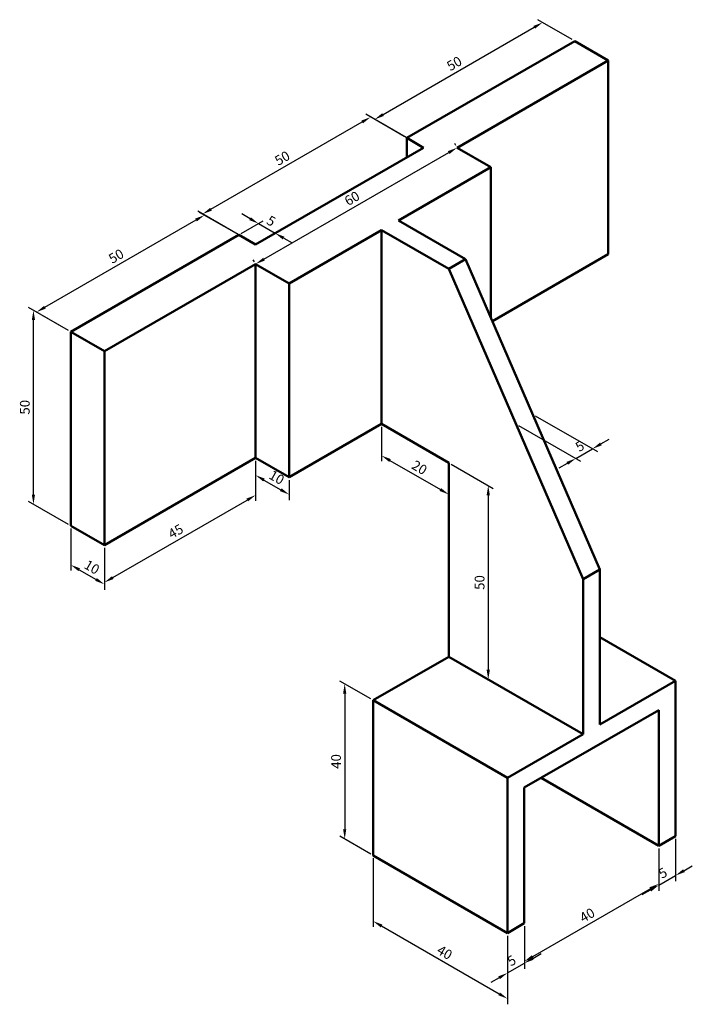
# Model space of a CAD drawing. Units: millimetres. Extents: x 2718 to 2891, y 1466 to 1720.
import ezdxf

# ---------------------------------------------------------------- set-up
doc = ezdxf.new("R2010")
doc.units = ezdxf.units.MM
doc.layers.add('M-DIMS', color=2, linetype='Continuous', lineweight=25)
doc.layers.add('M-OUTL', color=7, linetype='Continuous', lineweight=50)
doc.styles.get("Standard").update_dxf_attribs({"font": 'arial.ttf'})
doc.dimstyles.new('ISO-25', dxfattribs={"dimtxt": 2.5, "dimasz": 2.5, "dimexe": 1.25, "dimexo": 0.625, "dimtad": 1, "dimtxsty": 'Standard', "dimcen": 2.5, "dimadec": 0, "dimazin": 0, "dimtfac": 1, "dimtmove": 0, "dimatfit": 3, "dimfxl": 1, "dimarcsym": 0})

# ---------------------------------------------------------------- blocks, each defined once
blk = doc.blocks.new('*D1')
at = {"layer": 'Defpoints', "color": 0, "transparency": 16777216}
for p in [(2808.89, 1504.71), (2843.54, 1484.71), (2843.54, 1467.77)]:
    blk.add_point(p, dxfattribs=at)
at = {"layer": 'M-DIMS', "color": 0, "lineweight": -2, "transparency": 16777216}
for p, q in [((2808.89, 1503.99), (2808.89, 1486.33)), ((2811.06, 1486.52), (2841.37, 1469.02)), ((2843.54, 1483.99), (2843.54, 1466.33))]:
    blk.add_line(p, q, dxfattribs=at)
at = {"layer": 'M-DIMS', "color": 0, "transparency": 16777216}
for points in [[(2811.27, 1486.88), (2810.85, 1486.16), (2808.89, 1487.77)], [(2841.58, 1469.38), (2841.16, 1468.66), (2843.54, 1467.77)]]:
    blk.add_solid(points, dxfattribs=at)
at = {"layer": 'M-DIMS', "color": 0, "transparency": 16777216, "insert": (2827.17, 1479.42), "char_height": 2.5, "attachment_point": 5, "rotation": 330}
blk.add_mtext('40', dxfattribs=at)
blk = doc.blocks.new('*D2')
at = {"layer": 'Defpoints', "color": 0, "transparency": 16777216}
for p in [(2847.87, 1487.21), (2843.54, 1484.71), (2847.87, 1476.93)]:
    blk.add_point(p, dxfattribs=at)
at = {"layer": 'M-DIMS', "color": 0, "lineweight": -2, "transparency": 16777216}
for p, q in [((2847.87, 1486.49), (2847.87, 1475.49)), ((2843.54, 1483.99), (2843.54, 1472.99)), ((2850.03, 1478.18), (2852.2, 1479.43)), ((2843.54, 1474.43), (2847.87, 1476.93)), ((2841.37, 1473.18), (2839.21, 1471.93))]:
    blk.add_line(p, q, dxfattribs=at)
at = {"layer": 'M-DIMS', "color": 0, "transparency": 16777216}
for points in [[(2849.82, 1478.54), (2850.24, 1477.82), (2847.87, 1476.93)], [(2841.16, 1473.54), (2841.58, 1472.82), (2843.54, 1474.43)]]:
    blk.add_solid(points, dxfattribs=at)
at = {"layer": 'M-DIMS', "color": 0, "transparency": 16777216, "insert": (2844.75, 1477.32), "char_height": 2.5, "attachment_point": 5, "rotation": 30}
blk.add_mtext('5', dxfattribs=at)
blk = doc.blocks.new('*D3')
at = {"layer": 'Defpoints', "color": 0, "transparency": 16777216}
for p in [(2882.51, 1507.21), (2882.51, 1497.39), (2847.87, 1487.21)]:
    blk.add_point(p, dxfattribs=at)
at = {"layer": 'M-DIMS', "color": 0, "lineweight": -2, "transparency": 16777216}
for p, q in [((2882.51, 1506.49), (2882.51, 1495.95)), ((2850.03, 1478.64), (2880.34, 1496.14)), ((2847.87, 1486.49), (2847.87, 1475.95))]:
    blk.add_line(p, q, dxfattribs=at)
at = {"layer": 'M-DIMS', "color": 0, "transparency": 16777216}
for points in [[(2880.13, 1496.5), (2880.55, 1495.78), (2882.51, 1497.39)], [(2849.82, 1479), (2850.24, 1478.28), (2847.87, 1477.39)]]:
    blk.add_solid(points, dxfattribs=at)
at = {"layer": 'M-DIMS', "color": 0, "transparency": 16777216, "insert": (2864.24, 1489.04), "char_height": 2.5, "attachment_point": 5, "rotation": 30}
blk.add_mtext('40', dxfattribs=at)
blk = doc.blocks.new('*D4')
at = {"layer": 'Defpoints', "color": 0, "transparency": 16777216}
for p in [(2886.84, 1509.71), (2882.51, 1507.21), (2886.84, 1499.53)]:
    blk.add_point(p, dxfattribs=at)
at = {"layer": 'M-DIMS', "color": 0, "lineweight": -2, "transparency": 16777216}
for p, q in [((2886.84, 1508.99), (2886.84, 1498.08)), ((2882.51, 1506.49), (2882.51, 1495.58)), ((2889, 1500.78), (2891.17, 1502.03)), ((2882.51, 1497.03), (2886.84, 1499.53)), ((2880.34, 1495.78), (2878.18, 1494.53))]:
    blk.add_line(p, q, dxfattribs=at)
at = {"layer": 'M-DIMS', "color": 0, "transparency": 16777216}
for points in [[(2888.79, 1501.14), (2889.21, 1500.42), (2886.84, 1499.53)], [(2880.13, 1496.14), (2880.55, 1495.42), (2882.51, 1497.03)]]:
    blk.add_solid(points, dxfattribs=at)
at = {"layer": 'M-DIMS', "color": 0, "transparency": 16777216, "insert": (2883.72, 1499.92), "char_height": 2.5, "attachment_point": 5, "rotation": 30}
blk.add_mtext('5', dxfattribs=at)
blk = doc.blocks.new('*D5')
at = {"layer": 'Defpoints', "color": 0, "transparency": 16777216}
for p in [(2828.38, 1605.96), (2828.38, 1555.96), (2838.56, 1550.09)]:
    blk.add_point(p, dxfattribs=at)
at = {"layer": 'M-DIMS', "color": 0, "lineweight": -2, "transparency": 16777216}
for p, q in [((2829.01, 1605.6), (2839.81, 1599.36)), ((2838.56, 1597.59), (2838.56, 1552.59)), ((2829.01, 1555.6), (2839.81, 1549.36))]:
    blk.add_line(p, q, dxfattribs=at)
at = {"layer": 'M-DIMS', "color": 0, "transparency": 16777216}
for points in [[(2838.15, 1597.59), (2838.98, 1597.59), (2838.56, 1600.09)], [(2838.15, 1552.59), (2838.98, 1552.59), (2838.56, 1550.09)]]:
    blk.add_solid(points, dxfattribs=at)
at = {"layer": 'M-DIMS', "color": 0, "transparency": 16777216, "insert": (2836.66, 1575.09), "char_height": 2.5, "attachment_point": 5, "rotation": 90}
blk.add_mtext('50', dxfattribs=at)
blk = doc.blocks.new('*D6')
at = {"layer": 'Defpoints', "color": 0, "transparency": 16777216}
for p in [(2811.06, 1615.96), (2828.38, 1605.96), (2828.38, 1597.81)]:
    blk.add_point(p, dxfattribs=at)
at = {"layer": 'M-DIMS', "color": 0, "lineweight": -2, "transparency": 16777216}
for p, q in [((2811.06, 1615.24), (2811.06, 1606.37)), ((2813.22, 1606.56), (2826.22, 1599.06)), ((2828.38, 1605.24), (2828.38, 1596.37))]:
    blk.add_line(p, q, dxfattribs=at)
at = {"layer": 'M-DIMS', "color": 0, "transparency": 16777216}
for points in [[(2813.43, 1606.92), (2813.02, 1606.2), (2811.06, 1607.81)], [(2826.42, 1599.42), (2826.01, 1598.7), (2828.38, 1597.81)]]:
    blk.add_solid(points, dxfattribs=at)
at = {"layer": 'M-DIMS', "color": 0, "transparency": 16777216, "insert": (2820.67, 1604.46), "char_height": 2.5, "attachment_point": 5, "rotation": 330}
blk.add_mtext('20', dxfattribs=at)
blk = doc.blocks.new('*D7')
at = {"layer": 'Defpoints', "color": 0, "transparency": 16777216}
for p in [(2830.55, 1687.21), (2830.55, 1687.21), (2778.58, 1657.21)]:
    blk.add_point(p, dxfattribs=at)
at = {"layer": 'M-DIMS', "color": 0, "lineweight": -2, "transparency": 16777216}
for p, q in [((2780.75, 1658.46), (2828.38, 1685.96)), ((2830.23, 1687.76), (2829.92, 1688.3)), ((2778.27, 1657.76), (2777.96, 1658.3))]:
    blk.add_line(p, q, dxfattribs=at)
at = {"layer": 'M-DIMS', "color": 0, "transparency": 16777216}
for points in [[(2828.17, 1686.32), (2828.59, 1685.6), (2830.55, 1687.21)], [(2780.54, 1658.82), (2780.96, 1658.1), (2778.58, 1657.21)]]:
    blk.add_solid(points, dxfattribs=at)
at = {"layer": 'M-DIMS', "color": 0, "transparency": 16777216, "insert": (2803.61, 1673.86), "char_height": 2.5, "attachment_point": 5, "rotation": 30}
blk.add_mtext('60', dxfattribs=at)
blk = doc.blocks.new('*D8')
at = {"layer": 'Defpoints', "color": 0, "transparency": 16777216}
for p in [(2778.58, 1607.21), (2787.24, 1602.21), (2787.24, 1597.77)]:
    blk.add_point(p, dxfattribs=at)
at = {"layer": 'M-DIMS', "color": 0, "lineweight": -2, "transparency": 16777216}
for p, q in [((2778.58, 1606.49), (2778.58, 1601.33)), ((2780.75, 1601.52), (2785.08, 1599.02)), ((2787.24, 1601.49), (2787.24, 1596.33))]:
    blk.add_line(p, q, dxfattribs=at)
at = {"layer": 'M-DIMS', "color": 0, "transparency": 16777216}
for points in [[(2780.96, 1601.88), (2780.54, 1601.16), (2778.58, 1602.77)], [(2785.29, 1599.38), (2784.87, 1598.66), (2787.24, 1597.77)]]:
    blk.add_solid(points, dxfattribs=at)
at = {"layer": 'M-DIMS', "color": 0, "transparency": 16777216, "insert": (2783.86, 1601.92), "char_height": 2.5, "attachment_point": 5, "rotation": 330}
blk.add_mtext('10', dxfattribs=at)
blk = doc.blocks.new('*D9')
at = {"layer": 'Defpoints', "color": 0, "transparency": 16777216}
for p in [(2778.58, 1607.21), (2778.58, 1597.61), (2739.61, 1584.71)]:
    blk.add_point(p, dxfattribs=at)
at = {"layer": 'M-DIMS', "color": 0, "lineweight": -2, "transparency": 16777216}
for p, q in [((2778.58, 1606.49), (2778.58, 1596.16)), ((2741.78, 1576.36), (2776.42, 1596.36)), ((2739.61, 1583.99), (2739.61, 1573.66))]:
    blk.add_line(p, q, dxfattribs=at)
at = {"layer": 'M-DIMS', "color": 0, "transparency": 16777216}
for points in [[(2776.21, 1596.72), (2776.63, 1596), (2778.58, 1597.61)], [(2741.57, 1576.72), (2741.99, 1576), (2739.61, 1575.11)]]:
    blk.add_solid(points, dxfattribs=at)
at = {"layer": 'M-DIMS', "color": 0, "transparency": 16777216, "insert": (2758.15, 1588), "char_height": 2.5, "attachment_point": 5, "rotation": 30}
blk.add_mtext('45', dxfattribs=at)
blk = doc.blocks.new('*D10')
at = {"layer": 'Defpoints', "color": 0, "transparency": 16777216}
for p in [(2730.95, 1589.71), (2739.61, 1584.71), (2739.61, 1574.64)]:
    blk.add_point(p, dxfattribs=at)
at = {"layer": 'M-DIMS', "color": 0, "lineweight": -2, "transparency": 16777216}
for p, q in [((2730.95, 1588.99), (2730.95, 1578.19)), ((2739.61, 1583.99), (2739.61, 1573.19)), ((2733.12, 1578.39), (2737.45, 1575.89))]:
    blk.add_line(p, q, dxfattribs=at)
at = {"layer": 'M-DIMS', "color": 0, "transparency": 16777216}
for points in [[(2733.33, 1578.75), (2732.91, 1578.03), (2730.95, 1579.64)], [(2737.66, 1576.25), (2737.24, 1575.53), (2739.61, 1574.64)]]:
    blk.add_solid(points, dxfattribs=at)
at = {"layer": 'M-DIMS', "color": 0, "transparency": 16777216, "insert": (2736.23, 1578.78), "char_height": 2.5, "attachment_point": 5, "rotation": 330}
blk.add_mtext('10', dxfattribs=at)
blk = doc.blocks.new('*D11')
at = {"layer": 'Defpoints', "color": 0, "transparency": 16777216}
for p in [(2721.32, 1645.28), (2730.95, 1639.71), (2730.95, 1589.71)]:
    blk.add_point(p, dxfattribs=at)
at = {"layer": 'M-DIMS', "color": 0, "lineweight": -2, "transparency": 16777216}
for p, q in [((2730.33, 1640.07), (2720.07, 1646)), ((2721.32, 1597.78), (2721.32, 1642.78)), ((2730.33, 1590.07), (2720.07, 1596))]:
    blk.add_line(p, q, dxfattribs=at)
at = {"layer": 'M-DIMS', "color": 0, "transparency": 16777216}
for points in [[(2720.9, 1642.78), (2721.73, 1642.78), (2721.32, 1645.28)], [(2720.9, 1597.78), (2721.73, 1597.78), (2721.32, 1595.28)]]:
    blk.add_solid(points, dxfattribs=at)
at = {"layer": 'M-DIMS', "color": 0, "transparency": 16777216, "insert": (2719.42, 1620.28), "char_height": 2.5, "attachment_point": 5, "rotation": 90}
blk.add_mtext('50', dxfattribs=at)
blk = doc.blocks.new('*D12')
at = {"layer": 'Defpoints', "color": 0, "transparency": 16777216}
for p in [(2765.41, 1669.82), (2774.25, 1664.71), (2730.95, 1639.71)]:
    blk.add_point(p, dxfattribs=at)
at = {"layer": 'M-DIMS', "color": 0, "lineweight": -2, "transparency": 16777216}
for p, q in [((2724.27, 1646.07), (2763.24, 1668.57)), ((2773.63, 1665.07), (2764.16, 1670.54)), ((2730.33, 1640.07), (2720.86, 1645.54))]:
    blk.add_line(p, q, dxfattribs=at)
at = {"layer": 'M-DIMS', "color": 0, "transparency": 16777216}
for points in [[(2763.03, 1668.93), (2763.45, 1668.21), (2765.41, 1669.82)], [(2724.06, 1646.43), (2724.48, 1645.71), (2722.11, 1644.82)]]:
    blk.add_solid(points, dxfattribs=at)
at = {"layer": 'M-DIMS', "color": 0, "transparency": 16777216, "insert": (2742.81, 1658.97), "char_height": 2.5, "attachment_point": 5, "rotation": 30}
blk.add_mtext('50', dxfattribs=at)
blk = doc.blocks.new('*D13')
at = {"layer": 'Defpoints', "color": 0, "transparency": 16777216}
for p in [(2774.25, 1664.71), (2783.66, 1665.14), (2778.58, 1662.21)]:
    blk.add_point(p, dxfattribs=at)
at = {"layer": 'M-DIMS', "color": 0, "lineweight": -2, "transparency": 16777216}
for p, q in [((2774.88, 1665.07), (2780.58, 1668.37)), ((2777.17, 1668.89), (2775, 1670.14)), ((2779.21, 1662.57), (2784.91, 1665.87)), ((2779.33, 1667.64), (2783.66, 1665.14)), ((2785.83, 1663.89), (2787.99, 1662.64))]:
    blk.add_line(p, q, dxfattribs=at)
at = {"layer": 'M-DIMS', "color": 0, "transparency": 16777216}
for points in [[(2777.37, 1669.26), (2776.96, 1668.53), (2779.33, 1667.64)], [(2786.03, 1664.26), (2785.62, 1663.53), (2783.66, 1665.14)]]:
    blk.add_solid(points, dxfattribs=at)
at = {"layer": 'M-DIMS', "color": 0, "transparency": 16777216, "insert": (2782.44, 1668.04), "char_height": 2.5, "attachment_point": 5, "rotation": 330}
blk.add_mtext('5', dxfattribs=at)
blk = doc.blocks.new('*D14')
at = {"layer": 'Defpoints', "color": 0, "transparency": 16777216}
for p in [(2808.23, 1695.1), (2821.89, 1687.21), (2778.58, 1662.21)]:
    blk.add_point(p, dxfattribs=at)
at = {"layer": 'M-DIMS', "color": 0, "lineweight": -2, "transparency": 16777216}
for p, q in [((2767.09, 1671.35), (2806.07, 1693.85)), ((2821.26, 1687.57), (2806.98, 1695.82)), ((2777.96, 1662.57), (2763.68, 1670.82))]:
    blk.add_line(p, q, dxfattribs=at)
at = {"layer": 'M-DIMS', "color": 0, "transparency": 16777216}
for points in [[(2805.86, 1694.21), (2806.27, 1693.49), (2808.23, 1695.1)], [(2766.89, 1671.71), (2767.3, 1670.99), (2764.93, 1670.1)]]:
    blk.add_solid(points, dxfattribs=at)
at = {"layer": 'M-DIMS', "color": 0, "transparency": 16777216, "insert": (2785.63, 1684.24), "char_height": 2.5, "attachment_point": 5, "rotation": 30}
blk.add_mtext('50', dxfattribs=at)
blk = doc.blocks.new('*D15')
at = {"layer": 'Defpoints', "color": 0, "transparency": 16777216}
for p in [(2852.57, 1719.5), (2860.86, 1714.71), (2817.56, 1689.71)]:
    blk.add_point(p, dxfattribs=at)
at = {"layer": 'M-DIMS', "color": 0, "lineweight": -2, "transparency": 16777216}
for p, q in [((2860.23, 1715.07), (2851.32, 1720.22)), ((2811.44, 1695.75), (2850.41, 1718.25)), ((2816.93, 1690.07), (2808.02, 1695.22))]:
    blk.add_line(p, q, dxfattribs=at)
at = {"layer": 'M-DIMS', "color": 0, "transparency": 16777216}
for points in [[(2850.2, 1718.61), (2850.62, 1717.89), (2852.57, 1719.5)], [(2811.23, 1696.11), (2811.65, 1695.39), (2809.27, 1694.5)]]:
    blk.add_solid(points, dxfattribs=at)
at = {"layer": 'M-DIMS', "color": 0, "transparency": 16777216, "insert": (2829.97, 1708.64), "char_height": 2.5, "attachment_point": 5, "rotation": 30}
blk.add_mtext('50', dxfattribs=at)
blk = doc.blocks.new('*D16')
at = {"layer": 'Defpoints', "color": 0, "transparency": 16777216}
for p in [(2850.03, 1618.46), (2845.7, 1615.96), (2865.44, 1609.57)]:
    blk.add_point(p, dxfattribs=at)
at = {"layer": 'M-DIMS', "color": 0, "lineweight": -2, "transparency": 16777216}
for p, q in [((2850.66, 1618.1), (2866.69, 1608.85)), ((2846.33, 1615.6), (2862.36, 1606.35)), ((2867.61, 1610.82), (2869.77, 1612.07)), ((2861.11, 1607.07), (2865.44, 1609.57)), ((2858.95, 1605.82), (2856.78, 1604.57))]:
    blk.add_line(p, q, dxfattribs=at)
at = {"layer": 'M-DIMS', "color": 0, "transparency": 16777216}
for points in [[(2867.4, 1611.18), (2867.81, 1610.46), (2865.44, 1609.57)], [(2858.74, 1606.18), (2859.15, 1605.46), (2861.11, 1607.07)]]:
    blk.add_solid(points, dxfattribs=at)
at = {"layer": 'M-DIMS', "color": 0, "transparency": 16777216, "insert": (2862.33, 1609.96), "char_height": 2.5, "attachment_point": 5, "rotation": 30}
blk.add_mtext('5', dxfattribs=at)
blk = doc.blocks.new('*D17')
at = {"layer": 'Defpoints', "color": 0, "transparency": 16777216}
for p in [(2808.89, 1544.71), (2801.56, 1508.95), (2808.89, 1504.71)]:
    blk.add_point(p, dxfattribs=at)
at = {"layer": 'M-DIMS', "color": 0, "lineweight": -2, "transparency": 16777216}
for p, q in [((2808.27, 1545.07), (2800.31, 1549.67)), ((2801.56, 1546.45), (2801.56, 1511.45)), ((2808.27, 1505.07), (2800.31, 1509.67))]:
    blk.add_line(p, q, dxfattribs=at)
at = {"layer": 'M-DIMS', "color": 0, "transparency": 16777216}
for points in [[(2801.14, 1546.45), (2801.97, 1546.45), (2801.56, 1548.95)], [(2801.14, 1511.45), (2801.97, 1511.45), (2801.56, 1508.95)]]:
    blk.add_solid(points, dxfattribs=at)
at = {"layer": 'M-DIMS', "color": 0, "transparency": 16777216, "insert": (2799.65, 1528.95), "char_height": 2.5, "attachment_point": 5, "rotation": 90}
blk.add_mtext('40', dxfattribs=at)

msp = doc.modelspace()

# ---------------------------------------------------------------- linework, layer by layer
at = {"layer": 'M-OUTL'}
for p, q in [((2817.555, 1689.714), (2860.856, 1714.714)), ((2860.856, 1714.714), (2869.517, 1709.714)), ((2869.517, 1709.714), (2830.545, 1687.214)), ((2869.517, 1709.714), (2869.517, 1659.714)), ((2821.885, 1687.214), (2817.555, 1689.714)), ((2817.555, 1684.714), (2817.555, 1689.714)), ((2778.584, 1662.214), (2821.885, 1687.214)), ((2830.545, 1687.214), (2839.206, 1682.214)), ((2815.39, 1668.464), (2839.206, 1682.214)), ((2839.206, 1682.214), (2839.206, 1643.464)), ((2832.711, 1658.464), (2815.39, 1668.464)), ((2787.244, 1652.214), (2811.06, 1665.964)), ((2811.06, 1665.964), (2811.06, 1615.964)), ((2811.06, 1665.964), (2828.38, 1655.964)), ((2730.953, 1639.714), (2774.254, 1664.714)), ((2774.254, 1664.714), (2778.584, 1662.214)), ((2828.38, 1655.964), (2832.711, 1658.464)), ((2832.711, 1658.464), (2867.352, 1578.464)), ((2869.517, 1659.714), (2839.639, 1642.464)), ((2739.613, 1634.714), (2778.584, 1657.214)), ((2778.584, 1657.214), (2787.244, 1652.214)), ((2778.584, 1657.214), (2778.584, 1607.214)), ((2828.38, 1655.964), (2863.021, 1575.964)), ((2787.244, 1602.214), (2787.244, 1652.214)), ((2730.953, 1639.714), (2730.953, 1589.714)), ((2739.613, 1634.714), (2730.953, 1639.714)), ((2739.613, 1584.714), (2739.613, 1634.714)), ((2811.06, 1615.964), (2787.244, 1602.214)), ((2811.06, 1615.964), (2828.38, 1605.964)), ((2778.584, 1607.214), (2739.613, 1584.714)), ((2778.584, 1607.214), (2787.244, 1602.214)), ((2828.38, 1605.964), (2828.38, 1555.964)), ((2730.953, 1589.714), (2739.613, 1584.714)), ((2867.352, 1578.464), (2863.021, 1575.964)), ((2867.352, 1538.464), (2867.352, 1578.464)), ((2863.021, 1575.964), (2863.021, 1535.964)), ((2886.837, 1549.714), (2867.352, 1560.964)), ((2828.38, 1555.964), (2808.895, 1544.714)), ((2863.021, 1535.964), (2828.38, 1555.964)), ((2886.837, 1549.714), (2867.352, 1538.464)), ((2886.837, 1509.714), (2886.837, 1549.714)), ((2808.895, 1544.714), (2808.895, 1504.714)), ((2843.536, 1524.714), (2808.895, 1544.714)), ((2847.866, 1522.214), (2882.507, 1542.214)), ((2882.507, 1542.214), (2882.507, 1507.214)), ((2843.536, 1524.714), (2863.021, 1535.964)), ((2843.536, 1484.714), (2843.536, 1524.714)), ((2882.507, 1507.214), (2852.196, 1524.714)), ((2847.866, 1487.214), (2847.866, 1522.214)), ((2882.507, 1507.214), (2886.837, 1509.714)), ((2808.895, 1504.714), (2843.536, 1484.714)), ((2843.536, 1484.714), (2847.866, 1487.214))]:
    msp.add_line(p, q, dxfattribs=at)

# ---------------------------------------------------------------- dimensions: what is measured, and where the dimension line sits
at = {"layer": 'M-DIMS'}
for p1, p2, distance, picture, middle in [((2817.555, 1689.714), (2860.856, 1714.714), 8.283, '*D15', (2829.972, 1708.643)), ((2778.584, 1662.214), (2821.885, 1687.214), 13.654, '*D14', (2785.63, 1684.244)), ((2778.584, 1657.214), (2830.545, 1687.214), 0, '*D7', (2803.614, 1673.861)), ((2730.953, 1639.714), (2774.254, 1664.714), 8.846, '*D12', (2742.806, 1658.968)), ((2774.254, 1664.714), (2778.584, 1662.214), 5.077, '*D13', (2782.444, 1668.037)), ((2730.953, 1589.714), (2730.953, 1639.714), 9.636, '*D11', (2719.415, 1620.277)), ((2845.701, 1615.964), (2850.031, 1618.464), -15.41, '*D16', (2862.327, 1609.959)), ((2811.06, 1615.964), (2828.38, 1605.964), -7.06, '*D6', (2820.671, 1604.458)), ((2739.613, 1584.714), (2778.584, 1607.214), -8.32, '*D9', (2758.15, 1588)), ((2778.584, 1607.214), (2787.244, 1602.214), -3.849, '*D8', (2783.865, 1601.916)), ((2828.38, 1605.964), (2828.38, 1555.964), 10.182, '*D5', (2836.661, 1575.085)), ((2730.953, 1589.714), (2739.613, 1584.714), -8.726, '*D10', (2736.233, 1578.784)), ((2808.895, 1544.714), (2808.895, 1504.714), -7.34, '*D17', (2799.654, 1528.951)), ((2882.507, 1507.214), (2886.837, 1509.714), -8.822, '*D4', (2883.724, 1499.92)), ((2847.866, 1487.214), (2882.507, 1507.214), -8.509, '*D3', (2864.236, 1489.036)), ((2808.895, 1504.714), (2843.536, 1484.714), -14.673, '*D1', (2827.166, 1479.417)), ((2843.536, 1484.714), (2847.866, 1487.214), -8.905, '*D2', (2844.753, 1477.323))]:
    dim = msp.add_aligned_dim(p1=p1, p2=p2, distance=distance, dimstyle='ISO-25', override={"dimclrd": 0, "dimclre": 0, "dimclrt": 0}, dxfattribs=at)
    dim.commit()
    dim.dimension.update_dxf_attribs({"geometry": picture, "text_midpoint": middle})

doc.saveas('drawing.dxf')
